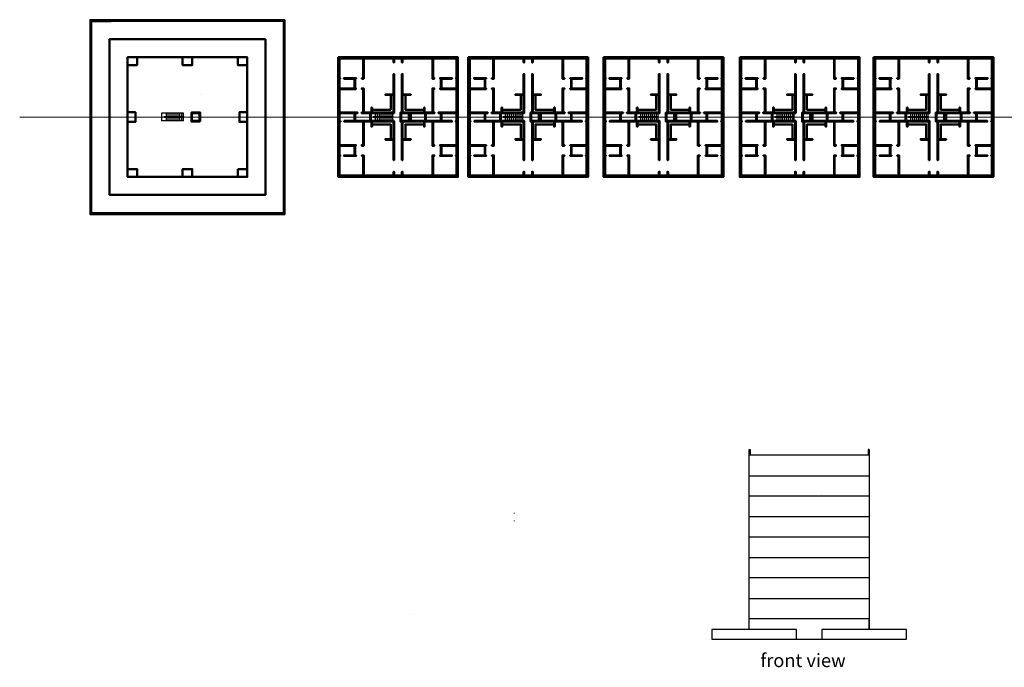
# Model space of a CAD drawing. Units: feet. Extents: x -1943 to 7856, y -1242 to 2749.
# Tile 1 of 2: x -1943 to 4124, y -1242 to 2749. Entities that reach past the tile are written whole.
import ezdxf

# ---------------------------------------------------------------- set-up
doc = ezdxf.new("R2010")
doc.units = ezdxf.units.FT
for name, color, linetype, lineweight in [('A-ANNO-SYMB', 1, 'Continuous', 18), ('A-ANNO-TEXT', 7, 'Continuous', 25), ('A-CONS', 8, 'Continuous', 13), ('A-ELEV', 7, 'Continuous', 25), ('A-FLOR-STRS', 3, 'Continuous', 25), ('A-WALL', 7, 'Continuous', 50), ('C-PROP', 6, 'Continuous', 35)]:
    doc.layers.add(name, color=color, linetype=linetype, lineweight=lineweight)
doc.styles.get("Standard").update_dxf_attribs({"font": 'arial.ttf'})

# ---------------------------------------------------------------- blocks, each defined once
blk = doc.blocks.new('STAIR')
for p, q in [((-933.2, 2172.8), (-1068.1, 2172.8)), ((-1068.1, 2172.8), (-1068.1, 2124.8)), ((-933.2, 2124.8), (-1068.1, 2124.8)), ((-1041.2, 2172.8), (-1041.2, 2151.4)), ((-1041.2, 2146.3), (-1041.2, 2124.8)), ((-1029.2, 2172.8), (-1029.2, 2151.4)), ((-1029.2, 2146.3), (-1029.2, 2124.8)), ((-1017.2, 2172.8), (-1017.2, 2151.4)), ((-1017.2, 2146.3), (-1017.2, 2124.8)), ((-1005.2, 2172.8), (-1005.2, 2151.4)), ((-1005.2, 2146.3), (-1005.2, 2124.8)), ((-993.2, 2172.8), (-993.2, 2151.4)), ((-993.2, 2146.3), (-993.2, 2124.8)), ((-981.2, 2172.8), (-981.2, 2151.4)), ((-981.2, 2146.3), (-981.2, 2124.8)), ((-969.2, 2172.8), (-969.2, 2151.4)), ((-969.2, 2146.3), (-969.2, 2124.8)), ((-957.2, 2172.8), (-957.2, 2151.4)), ((-957.2, 2146.3), (-957.2, 2124.8)), ((-945.2, 2172.8), (-945.2, 2151.4))]:
    blk.add_line(p, q)
for points in [[(-1053.2, 2151.4), (-933.2, 2151.4), (-933.2, 2146.3), (-1053.2, 2146.3)], [(-1052.2, 2150.4), (-934.2, 2150.4), (-934.2, 2147.3), (-1052.2, 2147.3)]]:
    blk.add_lwpolyline(points, close=True)
for points in [[(-945.2, 2146.3), (-945.2, 2124.8)], [(-933.2, 2124.8), (-933.2, 2172.8)]]:
    blk.add_lwpolyline(points)

msp = doc.modelspace()

# ---------------------------------------------------------------- linework, layer by layer
at = {"layer": 'A-ANNO-SYMB'}
msp.add_line((-1942.9, 2148.8), (7856.1, 2148.8), dxfattribs=at)
at = {"layer": 'A-CONS'}
for p, q in [((1105.6, -291.9, 260.8), (1101.6, -291.9, 260.8)), ((1105.6, -339.9, 260.8), (1101.6, -339.9, 260.8)), ((477.6, -915.9, 80.8), (477.6, -915.9, 140.8))]:
    msp.add_line(p, q, dxfattribs=at)
at = {"layer": 'A-ELEV'}
for p, q in [((2552.9, 100.4), (2558.9, 100.4)), ((2552.9, -1009.6), (2552.9, 100.4)), ((3290.9, 64.4), (2552.9, 64.4)), ((2558.9, 100.4), (2558.9, 64.4)), ((3290.9, 100.4), (3284.9, 100.4)), ((3284.9, 100.4), (3284.9, 64.4)), ((3290.9, 64.4), (3290.9, 100.4)), ((3290.9, 100.4), (3290.9, -1009.6)), ((2552.9, -61.6), (3290.9, -61.6)), ((3000, -175.9), (3000, -175.9)), ((3290.9, -187.6), (2552.9, -187.6)), ((2552.9, -313.6), (3290.9, -313.6)), ((3290.9, -439.6), (2552.9, -439.6)), ((3290.9, -439.6), (2552.9, -439.6)), ((2552.9, -565.6), (3290.9, -565.6)), ((3290.9, -691.6), (2552.9, -691.6)), ((2552.9, -817.6), (3290.9, -817.6)), ((3290.9, -943.6), (2552.9, -943.6)), ((3290.9, -1009.6), (3290.9, -949.6)), ((2844.1, -1009.6), (2321.9, -1009.6)), ((2321.9, -1009.6), (2321.9, -1069.6)), ((2844.1, -1069.6), (2844.1, -1009.6)), ((3521.9, -1009.6), (2999.8, -1009.6)), ((2999.8, -1009.6), (2999.8, -1069.6)), ((3521.9, -1069.6), (3521.9, -1009.6)), ((2321.9, -1069.6), (3521.9, -1069.6))]:
    msp.add_line(p, q, dxfattribs=at)
at = {"layer": 'A-WALL'}
for p, q in [((-1500.2, 2739.8), (-1380.2, 2739.8)), ((-1389.2, 2628.8), (-429.2, 2628.8)), ((-1389.2, 1668.8), (-1389.2, 2628.8)), ((-429.2, 2628.8), (-429.2, 1668.8)), ((-831.1, 2288.8), (-831.1, 2288.8)), ((466.6, 2288.8), (466.6, 2288.8)), ((1268.5, 2288.8), (1268.5, 2288.8)), ((2102.6, 2288.8), (2102.6, 2288.8)), ((2941.6, 2288.8), (2941.6, 2288.8)), ((3766, 2288.8), (3766, 2288.8)), ((-429.2, 1668.8), (-1389.2, 1668.8))]:
    msp.add_line(p, q, dxfattribs=at)
for points in [[(-429.2, 2628.8), (-429.2, 1668.8), (-1389.2, 1668.8), (-1389.2, 2628.8)], [(-540.2, 2517.8), (-540.2, 1779.8), (-1278.2, 1779.8), (-1278.2, 2517.8)], [(-1278.2, 2517.8), (-1219.1, 2517.8), (-1219.1, 2469.1), (-1278.2, 2469.1)], [(-938.7, 2517.8), (-879.6, 2517.8), (-879.6, 2469.1), (-938.7, 2469.1)], [(-599.2, 2517.8), (-540.2, 2517.8), (-540.2, 2469.1), (-599.2, 2469.1)], [(19.6, 2517.8), (19.6, 1779.8), (757.6, 1779.8), (757.6, 2517.8)], [(821.4, 2517.8), (821.4, 1779.8), (1559.4, 1779.8), (1559.4, 2517.8)], [(1655.5, 2517.8), (1655.5, 1779.8), (2393.5, 1779.8), (2393.5, 2517.8)], [(2494.5, 2517.8), (2494.5, 1779.8), (3232.5, 1779.8), (3232.5, 2517.8)], [(3319, 2517.8), (3319, 1779.8), (4057, 1779.8), (4057, 2517.8)], [(-1278.2, 2119.3), (-1278.2, 2178.4), (-1229.4, 2178.4), (-1229.4, 2119.3)], [(-830.6, 2120.8), (-885.2, 2120.8), (-885.2, 2176.8), (-830.6, 2176.8)], [(-834.6, 2124.8), (-881.2, 2124.8), (-881.2, 2172.8), (-834.6, 2172.8)], [(-540.2, 2178.4), (-540.2, 2119.3), (-588.9, 2119.3), (-588.9, 2178.4)], [(458.1, 2120.8), (403.5, 2120.8), (403.5, 2176.8), (458.1, 2176.8)], [(454.1, 2124.8), (407.5, 2124.8), (407.5, 2172.8), (454.1, 2172.8)], [(1260, 2120.8), (1205.3, 2120.8), (1205.3, 2176.8), (1260, 2176.8)], [(1256, 2124.8), (1209.3, 2124.8), (1209.3, 2172.8), (1256, 2172.8)], [(2094.1, 2120.8), (2039.5, 2120.8), (2039.5, 2176.8), (2094.1, 2176.8)], [(2090.1, 2124.8), (2043.5, 2124.8), (2043.5, 2172.8), (2090.1, 2172.8)], [(2933.1, 2120.8), (2878.5, 2120.8), (2878.5, 2176.8), (2933.1, 2176.8)], [(2929.1, 2124.8), (2882.5, 2124.8), (2882.5, 2172.8), (2929.1, 2172.8)], [(3757.5, 2120.8), (3702.9, 2120.8), (3702.9, 2176.8), (3757.5, 2176.8)], [(3753.5, 2124.8), (3706.9, 2124.8), (3706.9, 2172.8), (3753.5, 2172.8)], [(-1278.2, 1828.6), (-1219.1, 1828.6), (-1219.1, 1779.8), (-1278.2, 1779.8)], [(-879.6, 1779.8), (-938.7, 1779.8), (-938.7, 1828.6), (-879.6, 1828.6)], [(-599.2, 1828.6), (-540.2, 1828.6), (-540.2, 1779.8), (-599.2, 1779.8)]]:
    msp.add_lwpolyline(points, close=True, dxfattribs=at)
for points in [[(560.6, 2124.8), (652.6, 2124.8), (652.6, 2172.8), (637.7, 2172.8), (637.7, 2176.8), (748.6, 2176.8), (748.6, 2321.3), (647.8, 2321.3), (647.8, 2325.3), (652.6, 2325.3), (652.6, 2384.8), (647.5, 2384.8), (647.5, 2388.8), (722, 2388.8), (722, 2384.8), (656.6, 2384.8), (656.6, 2325.3), (748.6, 2325.3), (748.6, 2384.8), (746, 2384.8), (746, 2388.8), (748.6, 2388.8), (748.6, 2508.8), (604.1, 2508.8), (604.1, 2388.8), (611.5, 2388.8), (611.5, 2384.8), (600.1, 2384.8), (600.1, 2508.8), (416.6, 2508.8), (416.6, 2485.7), (412.6, 2485.7), (412.6, 2508.8), (364.6, 2508.8), (364.6, 2485.7), (360.6, 2485.7), (360.6, 2508.8), (177.1, 2508.8), (177.1, 2384.8), (165.6, 2384.8), (165.6, 2388.8), (173.1, 2388.8), (173.1, 2508.8), (28.6, 2508.8), (28.6, 2388.8), (31.1, 2388.8), (31.1, 2384.8), (28.6, 2384.8), (28.6, 2325.3), (120.6, 2325.3), (120.6, 2384.8), (55.1, 2384.8), (55.1, 2388.8), (129.6, 2388.8), (129.6, 2384.8), (124.6, 2384.8), (124.6, 2325.3), (129.4, 2325.3), (129.4, 2321.3), (28.6, 2321.3), (28.6, 2176.8), (139.5, 2176.8), (139.5, 2172.8), (124.6, 2172.8), (124.6, 2124.8), (216.6, 2124.8), (216.6, 2172.8), (216.6, 2124.8), (216.6, 2172.8), (163.5, 2172.8), (163.5, 2176.8), (173.1, 2176.8), (173.1, 2321.3), (165.4, 2321.3), (165.4, 2325.3), (177.1, 2325.3), (177.1, 2176.8), (224.6, 2176.8), (224.6, 2207.4), (228.6, 2207.4), (228.6, 2176.8), (360.6, 2176.8), (360.6, 2284.8), (310.5, 2284.8), (310.5, 2288.8), (360.6, 2288.8), (360.6, 2413.7), (364.6, 2413.7), (364.6, 2172.8), (220.6, 2172.8), (220.6, 2124.8), (364.6, 2124.8), (364.6, 1884), (360.6, 1884), (360.6, 2008.8), (310.5, 2008.8), (310.5, 2012.8), (360.6, 2012.8), (360.6, 2120.8), (228.6, 2120.8), (228.6, 2090.3), (224.6, 2090.3), (224.6, 2120.8), (177.1, 2120.8), (177.1, 1972.3), (165.4, 1972.3), (165.4, 1976.3), (173.1, 1976.3), (173.1, 2120.8), (57.1, 2120.8), (57.1, 2124.8), (120.6, 2124.8), (120.6, 2172.8), (28.6, 2172.8), (28.6, 2124.8), (33.1, 2124.8), (33.1, 2120.8), (28.6, 2120.8), (28.6, 1976.3), (129.4, 1976.3), (129.4, 1972.3), (124.6, 1972.3), (124.6, 1912.8), (129.6, 1912.8), (129.6, 1908.8), (56.5, 1908.8), (56.5, 1912.8), (120.6, 1912.8), (120.6, 1972.3), (28.6, 1972.3), (28.6, 1912.8), (32.5, 1912.8), (32.5, 1908.8), (28.6, 1908.8), (28.6, 1788.8), (173.1, 1788.8), (173.1, 1908.8), (165.6, 1908.8), (165.6, 1912.8), (177.1, 1912.8), (177.1, 1788.8), (360.6, 1788.8), (360.6, 1812), (364.6, 1812), (364.6, 1788.8), (412.6, 1788.8), (412.6, 1812), (416.6, 1812), (416.6, 1788.8), (600.1, 1788.8), (600.1, 1912.8), (611.5, 1912.8), (611.5, 1908.8), (604.1, 1908.8), (604.1, 1788.8), (748.6, 1788.8), (748.6, 1908.8), (744.7, 1908.8), (744.7, 1912.8), (748.6, 1912.8), (748.6, 1972.3), (656.6, 1972.3), (656.6, 1912.8), (720.7, 1912.8), (720.7, 1908.8), (647.5, 1908.8), (647.5, 1912.8), (652.6, 1912.8), (652.6, 1972.3), (647.8, 1972.3), (647.8, 1976.3), (748.6, 1976.3), (748.6, 2120.8), (744.1, 2120.8), (744.1, 2124.8), (748.6, 2124.8), (748.6, 2172.8), (656.6, 2172.8), (656.6, 2124.8), (720.1, 2124.8), (720.1, 2120.8), (604.1, 2120.8), (604.1, 1976.3), (611.8, 1976.3), (611.8, 1972.3), (600.1, 1972.3), (600.1, 2120.8), (552.6, 2120.8), (552.6, 2090.3), (548.6, 2090.3), (548.6, 2120.8), (416.6, 2120.8), (416.6, 2012.8), (466.6, 2012.8), (466.6, 2008.8), (416.6, 2008.8), (416.6, 1884), (412.6, 1884), (412.6, 2124.8), (463.2, 2124.8), (463.2, 2172.8), (412.6, 2172.8), (412.6, 2413.7), (416.6, 2413.7), (416.6, 2288.8), (466.6, 2288.8), (466.6, 2284.8), (416.6, 2284.8), (416.6, 2176.8), (548.6, 2176.8), (548.6, 2207.4), (552.6, 2207.4), (552.6, 2176.8), (600.1, 2176.8), (600.1, 2325.3), (611.8, 2325.3), (611.8, 2321.3), (604.1, 2321.3), (604.1, 2176.8), (613.7, 2176.8), (613.7, 2172.8), (560.6, 2172.8), (560.6, 2124.8), (560.6, 2172.8)], [(1362.4, 2124.8), (1454.4, 2124.8), (1454.4, 2172.8), (1439.5, 2172.8), (1439.5, 2176.8), (1550.4, 2176.8), (1550.4, 2321.3), (1449.6, 2321.3), (1449.6, 2325.3), (1454.4, 2325.3), (1454.4, 2384.8), (1449.3, 2384.8), (1449.3, 2388.8), (1523.8, 2388.8), (1523.8, 2384.8), (1458.4, 2384.8), (1458.4, 2325.3), (1550.4, 2325.3), (1550.4, 2384.8), (1547.8, 2384.8), (1547.8, 2388.8), (1550.4, 2388.8), (1550.4, 2508.8), (1405.9, 2508.8), (1405.9, 2388.8), (1413.3, 2388.8), (1413.3, 2384.8), (1401.9, 2384.8), (1401.9, 2508.8), (1218.4, 2508.8), (1218.4, 2485.7), (1214.4, 2485.7), (1214.4, 2508.8), (1166.4, 2508.8), (1166.4, 2485.7), (1162.4, 2485.7), (1162.4, 2508.8), (978.9, 2508.8), (978.9, 2384.8), (967.4, 2384.8), (967.4, 2388.8), (974.9, 2388.8), (974.9, 2508.8), (830.4, 2508.8), (830.4, 2388.8), (832.9, 2388.8), (832.9, 2384.8), (830.4, 2384.8), (830.4, 2325.3), (922.4, 2325.3), (922.4, 2384.8), (856.9, 2384.8), (856.9, 2388.8), (931.4, 2388.8), (931.4, 2384.8), (926.4, 2384.8), (926.4, 2325.3), (931.2, 2325.3), (931.2, 2321.3), (830.4, 2321.3), (830.4, 2176.8), (941.3, 2176.8), (941.3, 2172.8), (926.4, 2172.8), (926.4, 2124.8), (1018.4, 2124.8), (1018.4, 2172.8), (1018.4, 2124.8), (1018.4, 2172.8), (965.3, 2172.8), (965.3, 2176.8), (974.9, 2176.8), (974.9, 2321.3), (967.2, 2321.3), (967.2, 2325.3), (978.9, 2325.3), (978.9, 2176.8), (1026.4, 2176.8), (1026.4, 2207.4), (1030.4, 2207.4), (1030.4, 2176.8), (1162.4, 2176.8), (1162.4, 2284.8), (1112.3, 2284.8), (1112.3, 2288.8), (1162.4, 2288.8), (1162.4, 2413.7), (1166.4, 2413.7), (1166.4, 2172.8), (1022.4, 2172.8), (1022.4, 2124.8), (1166.4, 2124.8), (1166.4, 1884), (1162.4, 1884), (1162.4, 2008.8), (1112.3, 2008.8), (1112.3, 2012.8), (1162.4, 2012.8), (1162.4, 2120.8), (1030.4, 2120.8), (1030.4, 2090.3), (1026.4, 2090.3), (1026.4, 2120.8), (978.9, 2120.8), (978.9, 1972.3), (967.2, 1972.3), (967.2, 1976.3), (974.9, 1976.3), (974.9, 2120.8), (858.9, 2120.8), (858.9, 2124.8), (922.4, 2124.8), (922.4, 2172.8), (830.4, 2172.8), (830.4, 2124.8), (834.9, 2124.8), (834.9, 2120.8), (830.4, 2120.8), (830.4, 1976.3), (931.2, 1976.3), (931.2, 1972.3), (926.4, 1972.3), (926.4, 1912.8), (931.4, 1912.8), (931.4, 1908.8), (858.3, 1908.8), (858.3, 1912.8), (922.4, 1912.8), (922.4, 1972.3), (830.4, 1972.3), (830.4, 1912.8), (834.3, 1912.8), (834.3, 1908.8), (830.4, 1908.8), (830.4, 1788.8), (974.9, 1788.8), (974.9, 1908.8), (967.4, 1908.8), (967.4, 1912.8), (978.9, 1912.8), (978.9, 1788.8), (1162.4, 1788.8), (1162.4, 1812), (1166.4, 1812), (1166.4, 1788.8), (1214.4, 1788.8), (1214.4, 1812), (1218.4, 1812), (1218.4, 1788.8), (1401.9, 1788.8), (1401.9, 1912.8), (1413.3, 1912.8), (1413.3, 1908.8), (1405.9, 1908.8), (1405.9, 1788.8), (1550.4, 1788.8), (1550.4, 1908.8), (1546.5, 1908.8), (1546.5, 1912.8), (1550.4, 1912.8), (1550.4, 1972.3), (1458.4, 1972.3), (1458.4, 1912.8), (1522.5, 1912.8), (1522.5, 1908.8), (1449.3, 1908.8), (1449.3, 1912.8), (1454.4, 1912.8), (1454.4, 1972.3), (1449.6, 1972.3), (1449.6, 1976.3), (1550.4, 1976.3), (1550.4, 2120.8), (1545.9, 2120.8), (1545.9, 2124.8), (1550.4, 2124.8), (1550.4, 2172.8), (1458.4, 2172.8), (1458.4, 2124.8), (1521.9, 2124.8), (1521.9, 2120.8), (1405.9, 2120.8), (1405.9, 1976.3), (1413.6, 1976.3), (1413.6, 1972.3), (1401.9, 1972.3), (1401.9, 2120.8), (1354.4, 2120.8), (1354.4, 2090.3), (1350.4, 2090.3), (1350.4, 2120.8), (1218.4, 2120.8), (1218.4, 2012.8), (1268.5, 2012.8), (1268.5, 2008.8), (1218.4, 2008.8), (1218.4, 1884), (1214.4, 1884), (1214.4, 2124.8), (1265, 2124.8), (1265, 2172.8), (1214.4, 2172.8), (1214.4, 2413.7), (1218.4, 2413.7), (1218.4, 2288.8), (1268.5, 2288.8), (1268.5, 2284.8), (1218.4, 2284.8), (1218.4, 2176.8), (1350.4, 2176.8), (1350.4, 2207.4), (1354.4, 2207.4), (1354.4, 2176.8), (1401.9, 2176.8), (1401.9, 2325.3), (1413.6, 2325.3), (1413.6, 2321.3), (1405.9, 2321.3), (1405.9, 2176.8), (1415.5, 2176.8), (1415.5, 2172.8), (1362.4, 2172.8), (1362.4, 2124.8), (1362.4, 2172.8)], [(2196.5, 2124.8), (2288.5, 2124.8), (2288.5, 2172.8), (2273.6, 2172.8), (2273.6, 2176.8), (2384.5, 2176.8), (2384.5, 2321.3), (2283.7, 2321.3), (2283.7, 2325.3), (2288.5, 2325.3), (2288.5, 2384.8), (2283.5, 2384.8), (2283.5, 2388.8), (2358, 2388.8), (2358, 2384.8), (2292.5, 2384.8), (2292.5, 2325.3), (2384.5, 2325.3), (2384.5, 2384.8), (2382, 2384.8), (2382, 2388.8), (2384.5, 2388.8), (2384.5, 2508.8), (2240, 2508.8), (2240, 2388.8), (2247.5, 2388.8), (2247.5, 2384.8), (2236, 2384.8), (2236, 2508.8), (2052.5, 2508.8), (2052.5, 2485.7), (2048.5, 2485.7), (2048.5, 2508.8), (2000.5, 2508.8), (2000.5, 2485.7), (1996.5, 2485.7), (1996.5, 2508.8), (1813, 2508.8), (1813, 2384.8), (1801.6, 2384.8), (1801.6, 2388.8), (1809, 2388.8), (1809, 2508.8), (1664.5, 2508.8), (1664.5, 2388.8), (1667.1, 2388.8), (1667.1, 2384.8), (1664.5, 2384.8), (1664.5, 2325.3), (1756.5, 2325.3), (1756.5, 2384.8), (1691.1, 2384.8), (1691.1, 2388.8), (1765.6, 2388.8), (1765.6, 2384.8), (1760.5, 2384.8), (1760.5, 2325.3), (1765.4, 2325.3), (1765.4, 2321.3), (1664.5, 2321.3), (1664.5, 2176.8), (1775.4, 2176.8), (1775.4, 2172.8), (1760.5, 2172.8), (1760.5, 2124.8), (1852.5, 2124.8), (1852.5, 2172.8), (1852.5, 2124.8), (1852.5, 2172.8), (1799.4, 2172.8), (1799.4, 2176.8), (1809, 2176.8), (1809, 2321.3), (1801.4, 2321.3), (1801.4, 2325.3), (1813, 2325.3), (1813, 2176.8), (1860.5, 2176.8), (1860.5, 2207.4), (1864.5, 2207.4), (1864.5, 2176.8), (1996.5, 2176.8), (1996.5, 2284.8), (1946.5, 2284.8), (1946.5, 2288.8), (1996.5, 2288.8), (1996.5, 2413.7), (2000.5, 2413.7), (2000.5, 2172.8), (1856.5, 2172.8), (1856.5, 2124.8), (2000.5, 2124.8), (2000.5, 1884), (1996.5, 1884), (1996.5, 2008.8), (1946.5, 2008.8), (1946.5, 2012.8), (1996.5, 2012.8), (1996.5, 2120.8), (1864.5, 2120.8), (1864.5, 2090.3), (1860.5, 2090.3), (1860.5, 2120.8), (1813, 2120.8), (1813, 1972.3), (1801.4, 1972.3), (1801.4, 1976.3), (1809, 1976.3), (1809, 2120.8), (1693, 2120.8), (1693, 2124.8), (1756.5, 2124.8), (1756.5, 2172.8), (1664.5, 2172.8), (1664.5, 2124.8), (1669, 2124.8), (1669, 2120.8), (1664.5, 2120.8), (1664.5, 1976.3), (1765.4, 1976.3), (1765.4, 1972.3), (1760.5, 1972.3), (1760.5, 1912.8), (1765.6, 1912.8), (1765.6, 1908.8), (1692.4, 1908.8), (1692.4, 1912.8), (1756.5, 1912.8), (1756.5, 1972.3), (1664.5, 1972.3), (1664.5, 1912.8), (1668.4, 1912.8), (1668.4, 1908.8), (1664.5, 1908.8), (1664.5, 1788.8), (1809, 1788.8), (1809, 1908.8), (1801.6, 1908.8), (1801.6, 1912.8), (1813, 1912.8), (1813, 1788.8), (1996.5, 1788.8), (1996.5, 1812), (2000.5, 1812), (2000.5, 1788.8), (2048.5, 1788.8), (2048.5, 1812), (2052.5, 1812), (2052.5, 1788.8), (2236, 1788.8), (2236, 1912.8), (2247.5, 1912.8), (2247.5, 1908.8), (2240, 1908.8), (2240, 1788.8), (2384.5, 1788.8), (2384.5, 1908.8), (2380.6, 1908.8), (2380.6, 1912.8), (2384.5, 1912.8), (2384.5, 1972.3), (2292.5, 1972.3), (2292.5, 1912.8), (2356.6, 1912.8), (2356.6, 1908.8), (2283.5, 1908.8), (2283.5, 1912.8), (2288.5, 1912.8), (2288.5, 1972.3), (2283.7, 1972.3), (2283.7, 1976.3), (2384.5, 1976.3), (2384.5, 2120.8), (2380, 2120.8), (2380, 2124.8), (2384.5, 2124.8), (2384.5, 2172.8), (2292.5, 2172.8), (2292.5, 2124.8), (2356, 2124.8), (2356, 2120.8), (2240, 2120.8), (2240, 1976.3), (2247.7, 1976.3), (2247.7, 1972.3), (2236, 1972.3), (2236, 2120.8), (2188.5, 2120.8), (2188.5, 2090.3), (2184.5, 2090.3), (2184.5, 2120.8), (2052.5, 2120.8), (2052.5, 2012.8), (2102.6, 2012.8), (2102.6, 2008.8), (2052.5, 2008.8), (2052.5, 1884), (2048.5, 1884), (2048.5, 2124.8), (2099.1, 2124.8), (2099.1, 2172.8), (2048.5, 2172.8), (2048.5, 2413.7), (2052.5, 2413.7), (2052.5, 2288.8), (2102.6, 2288.8), (2102.6, 2284.8), (2052.5, 2284.8), (2052.5, 2176.8), (2184.5, 2176.8), (2184.5, 2207.4), (2188.5, 2207.4), (2188.5, 2176.8), (2236, 2176.8), (2236, 2325.3), (2247.7, 2325.3), (2247.7, 2321.3), (2240, 2321.3), (2240, 2176.8), (2249.6, 2176.8), (2249.6, 2172.8), (2196.5, 2172.8), (2196.5, 2124.8), (2196.5, 2172.8)], [(3035.5, 2124.8), (3127.5, 2124.8), (3127.5, 2172.8), (3112.6, 2172.8), (3112.6, 2176.8), (3223.5, 2176.8), (3223.5, 2321.3), (3122.7, 2321.3), (3122.7, 2325.3), (3127.5, 2325.3), (3127.5, 2384.8), (3122.5, 2384.8), (3122.5, 2388.8), (3197, 2388.8), (3197, 2384.8), (3131.5, 2384.8), (3131.5, 2325.3), (3223.5, 2325.3), (3223.5, 2384.8), (3221, 2384.8), (3221, 2388.8), (3223.5, 2388.8), (3223.5, 2508.8), (3079, 2508.8), (3079, 2388.8), (3086.5, 2388.8), (3086.5, 2384.8), (3075, 2384.8), (3075, 2508.8), (2891.5, 2508.8), (2891.5, 2485.7), (2887.5, 2485.7), (2887.5, 2508.8), (2839.5, 2508.8), (2839.5, 2485.7), (2835.5, 2485.7), (2835.5, 2508.8), (2652, 2508.8), (2652, 2384.8), (2640.6, 2384.8), (2640.6, 2388.8), (2648, 2388.8), (2648, 2508.8), (2503.5, 2508.8), (2503.5, 2388.8), (2506.1, 2388.8), (2506.1, 2384.8), (2503.5, 2384.8), (2503.5, 2325.3), (2595.5, 2325.3), (2595.5, 2384.8), (2530.1, 2384.8), (2530.1, 2388.8), (2604.6, 2388.8), (2604.6, 2384.8), (2599.5, 2384.8), (2599.5, 2325.3), (2604.4, 2325.3), (2604.4, 2321.3), (2503.5, 2321.3), (2503.5, 2176.8), (2614.4, 2176.8), (2614.4, 2172.8), (2599.5, 2172.8), (2599.5, 2124.8), (2691.5, 2124.8), (2691.5, 2172.8), (2691.5, 2124.8), (2691.5, 2172.8), (2638.4, 2172.8), (2638.4, 2176.8), (2648, 2176.8), (2648, 2321.3), (2640.4, 2321.3), (2640.4, 2325.3), (2652, 2325.3), (2652, 2176.8), (2699.5, 2176.8), (2699.5, 2207.4), (2703.5, 2207.4), (2703.5, 2176.8), (2835.5, 2176.8), (2835.5, 2284.8), (2785.5, 2284.8), (2785.5, 2288.8), (2835.5, 2288.8), (2835.5, 2413.7), (2839.5, 2413.7), (2839.5, 2172.8), (2695.5, 2172.8), (2695.5, 2124.8), (2839.5, 2124.8), (2839.5, 1884), (2835.5, 1884), (2835.5, 2008.8), (2785.5, 2008.8), (2785.5, 2012.8), (2835.5, 2012.8), (2835.5, 2120.8), (2703.5, 2120.8), (2703.5, 2090.3), (2699.5, 2090.3), (2699.5, 2120.8), (2652, 2120.8), (2652, 1972.3), (2640.4, 1972.3), (2640.4, 1976.3), (2648, 1976.3), (2648, 2120.8), (2532, 2120.8), (2532, 2124.8), (2595.5, 2124.8), (2595.5, 2172.8), (2503.5, 2172.8), (2503.5, 2124.8), (2508, 2124.8), (2508, 2120.8), (2503.5, 2120.8), (2503.5, 1976.3), (2604.4, 1976.3), (2604.4, 1972.3), (2599.5, 1972.3), (2599.5, 1912.8), (2604.6, 1912.8), (2604.6, 1908.8), (2531.4, 1908.8), (2531.4, 1912.8), (2595.5, 1912.8), (2595.5, 1972.3), (2503.5, 1972.3), (2503.5, 1912.8), (2507.4, 1912.8), (2507.4, 1908.8), (2503.5, 1908.8), (2503.5, 1788.8), (2648, 1788.8), (2648, 1908.8), (2640.6, 1908.8), (2640.6, 1912.8), (2652, 1912.8), (2652, 1788.8), (2835.5, 1788.8), (2835.5, 1812), (2839.5, 1812), (2839.5, 1788.8), (2887.5, 1788.8), (2887.5, 1812), (2891.5, 1812), (2891.5, 1788.8), (3075, 1788.8), (3075, 1912.8), (3086.5, 1912.8), (3086.5, 1908.8), (3079, 1908.8), (3079, 1788.8), (3223.5, 1788.8), (3223.5, 1908.8), (3219.6, 1908.8), (3219.6, 1912.8), (3223.5, 1912.8), (3223.5, 1972.3), (3131.5, 1972.3), (3131.5, 1912.8), (3195.6, 1912.8), (3195.6, 1908.8), (3122.5, 1908.8), (3122.5, 1912.8), (3127.5, 1912.8), (3127.5, 1972.3), (3122.7, 1972.3), (3122.7, 1976.3), (3223.5, 1976.3), (3223.5, 2120.8), (3219, 2120.8), (3219, 2124.8), (3223.5, 2124.8), (3223.5, 2172.8), (3131.5, 2172.8), (3131.5, 2124.8), (3195, 2124.8), (3195, 2120.8), (3079, 2120.8), (3079, 1976.3), (3086.7, 1976.3), (3086.7, 1972.3), (3075, 1972.3), (3075, 2120.8), (3027.5, 2120.8), (3027.5, 2090.3), (3023.5, 2090.3), (3023.5, 2120.8), (2891.5, 2120.8), (2891.5, 2012.8), (2941.6, 2012.8), (2941.6, 2008.8), (2891.5, 2008.8), (2891.5, 1884), (2887.5, 1884), (2887.5, 2124.8), (2938.1, 2124.8), (2938.1, 2172.8), (2887.5, 2172.8), (2887.5, 2413.7), (2891.5, 2413.7), (2891.5, 2288.8), (2941.6, 2288.8), (2941.6, 2284.8), (2891.5, 2284.8), (2891.5, 2176.8), (3023.5, 2176.8), (3023.5, 2207.4), (3027.5, 2207.4), (3027.5, 2176.8), (3075, 2176.8), (3075, 2325.3), (3086.7, 2325.3), (3086.7, 2321.3), (3079, 2321.3), (3079, 2176.8), (3088.6, 2176.8), (3088.6, 2172.8), (3035.5, 2172.8), (3035.5, 2124.8), (3035.5, 2172.8)], [(3860, 2124.8), (3952, 2124.8), (3952, 2172.8), (3937.1, 2172.8), (3937.1, 2176.8), (4048, 2176.8), (4048, 2321.3), (3947.1, 2321.3), (3947.1, 2325.3), (3952, 2325.3), (3952, 2384.8), (3946.9, 2384.8), (3946.9, 2388.8), (4021.4, 2388.8), (4021.4, 2384.8), (3956, 2384.8), (3956, 2325.3), (4048, 2325.3), (4048, 2384.8), (4045.4, 2384.8), (4045.4, 2388.8), (4048, 2388.8), (4048, 2508.8), (3903.5, 2508.8), (3903.5, 2388.8), (3910.9, 2388.8), (3910.9, 2384.8), (3899.5, 2384.8), (3899.5, 2508.8), (3716, 2508.8), (3716, 2485.7), (3712, 2485.7), (3712, 2508.8), (3664, 2508.8), (3664, 2485.7), (3660, 2485.7), (3660, 2508.8), (3476.5, 2508.8), (3476.5, 2384.8), (3465, 2384.8), (3465, 2388.8), (3472.5, 2388.8), (3472.5, 2508.8), (3328, 2508.8), (3328, 2388.8), (3330.5, 2388.8), (3330.5, 2384.8), (3328, 2384.8), (3328, 2325.3), (3420, 2325.3), (3420, 2384.8), (3354.5, 2384.8), (3354.5, 2388.8), (3429, 2388.8), (3429, 2384.8), (3424, 2384.8), (3424, 2325.3), (3428.8, 2325.3), (3428.8, 2321.3), (3328, 2321.3), (3328, 2176.8), (3438.8, 2176.8), (3438.8, 2172.8), (3424, 2172.8), (3424, 2124.8), (3516, 2124.8), (3516, 2172.8), (3516, 2124.8), (3516, 2172.8), (3462.8, 2172.8), (3462.8, 2176.8), (3472.5, 2176.8), (3472.5, 2321.3), (3464.8, 2321.3), (3464.8, 2325.3), (3476.5, 2325.3), (3476.5, 2176.8), (3524, 2176.8), (3524, 2207.4), (3528, 2207.4), (3528, 2176.8), (3660, 2176.8), (3660, 2284.8), (3609.9, 2284.8), (3609.9, 2288.8), (3660, 2288.8), (3660, 2413.7), (3664, 2413.7), (3664, 2172.8), (3520, 2172.8), (3520, 2124.8), (3664, 2124.8), (3664, 1884), (3660, 1884), (3660, 2008.8), (3609.9, 2008.8), (3609.9, 2012.8), (3660, 2012.8), (3660, 2120.8), (3528, 2120.8), (3528, 2090.3), (3524, 2090.3), (3524, 2120.8), (3476.5, 2120.8), (3476.5, 1972.3), (3464.8, 1972.3), (3464.8, 1976.3), (3472.5, 1976.3), (3472.5, 2120.8), (3356.5, 2120.8), (3356.5, 2124.8), (3420, 2124.8), (3420, 2172.8), (3328, 2172.8), (3328, 2124.8), (3332.5, 2124.8), (3332.5, 2120.8), (3328, 2120.8), (3328, 1976.3), (3428.8, 1976.3), (3428.8, 1972.3), (3424, 1972.3), (3424, 1912.8), (3429, 1912.8), (3429, 1908.8), (3355.9, 1908.8), (3355.9, 1912.8), (3420, 1912.8), (3420, 1972.3), (3328, 1972.3), (3328, 1912.8), (3331.9, 1912.8), (3331.9, 1908.8), (3328, 1908.8), (3328, 1788.8), (3472.5, 1788.8), (3472.5, 1908.8), (3465, 1908.8), (3465, 1912.8), (3476.5, 1912.8), (3476.5, 1788.8), (3660, 1788.8), (3660, 1812), (3664, 1812), (3664, 1788.8), (3712, 1788.8), (3712, 1812), (3716, 1812), (3716, 1788.8), (3899.5, 1788.8), (3899.5, 1912.8), (3910.9, 1912.8), (3910.9, 1908.8), (3903.5, 1908.8), (3903.5, 1788.8), (4048, 1788.8), (4048, 1908.8), (4044, 1908.8), (4044, 1912.8), (4048, 1912.8), (4048, 1972.3), (3956, 1972.3), (3956, 1912.8), (4020, 1912.8), (4020, 1908.8), (3946.9, 1908.8), (3946.9, 1912.8), (3952, 1912.8), (3952, 1972.3), (3947.1, 1972.3), (3947.1, 1976.3), (4048, 1976.3), (4048, 2120.8), (4043.5, 2120.8), (4043.5, 2124.8), (4048, 2124.8), (4048, 2172.8), (3956, 2172.8), (3956, 2124.8), (4019.5, 2124.8), (4019.5, 2120.8), (3903.5, 2120.8), (3903.5, 1976.3), (3911.1, 1976.3), (3911.1, 1972.3), (3899.5, 1972.3), (3899.5, 2120.8), (3852, 2120.8), (3852, 2090.3), (3848, 2090.3), (3848, 2120.8), (3716, 2120.8), (3716, 2012.8), (3766, 2012.8), (3766, 2008.8), (3716, 2008.8), (3716, 1884), (3712, 1884), (3712, 2124.8), (3762.6, 2124.8), (3762.6, 2172.8), (3712, 2172.8), (3712, 2413.7), (3716, 2413.7), (3716, 2288.8), (3766, 2288.8), (3766, 2284.8), (3716, 2284.8), (3716, 2176.8), (3848, 2176.8), (3848, 2207.4), (3852, 2207.4), (3852, 2176.8), (3899.5, 2176.8), (3899.5, 2325.3), (3911.1, 2325.3), (3911.1, 2321.3), (3903.5, 2321.3), (3903.5, 2176.8), (3913.1, 2176.8), (3913.1, 2172.8), (3860, 2172.8), (3860, 2124.8), (3860, 2172.8)], [(228.6, 2193.8), (343.6, 2193.8), (343.6, 2284.8)], [(548.6, 2193.8), (433.6, 2193.8), (433.6, 2284.8)], [(1030.4, 2193.8), (1145.4, 2193.8), (1145.4, 2284.8)], [(1350.4, 2193.8), (1235.4, 2193.8), (1235.4, 2284.8)], [(1864.5, 2193.8), (1979.6, 2193.8), (1979.6, 2284.8)], [(2184.5, 2193.8), (2069.5, 2193.8), (2069.5, 2284.8)], [(2703.5, 2193.8), (2818.5, 2193.8), (2818.5, 2284.8)], [(3023.5, 2193.8), (2908.5, 2193.8), (2908.5, 2284.8)], [(3528, 2193.8), (3643, 2193.8), (3643, 2284.8)], [(3848, 2193.8), (3732.9, 2193.8), (3732.9, 2284.8)], [(556.6, 2124.8), (467.2, 2124.8), (467.2, 2172.8), (556.6, 2172.8), (556.6, 2124.8), (556.6, 2172.8)], [(1358.4, 2124.8), (1269, 2124.8), (1269, 2172.8), (1358.4, 2172.8), (1358.4, 2124.8), (1358.4, 2172.8)], [(2192.5, 2124.8), (2103.1, 2124.8), (2103.1, 2172.8), (2192.5, 2172.8), (2192.5, 2124.8), (2192.5, 2172.8)], [(3031.5, 2124.8), (2942.1, 2124.8), (2942.1, 2172.8), (3031.5, 2172.8), (3031.5, 2124.8), (3031.5, 2172.8)], [(3856, 2124.8), (3766.6, 2124.8), (3766.6, 2172.8), (3856, 2172.8), (3856, 2124.8), (3856, 2172.8)], [(228.6, 2103.9), (343.6, 2103.9), (343.6, 2012.8)], [(548.6, 2103.9), (433.6, 2103.9), (433.6, 2012.8)], [(1030.4, 2103.9), (1145.4, 2103.9), (1145.4, 2012.8)], [(1350.4, 2103.9), (1235.4, 2103.9), (1235.4, 2012.8)], [(1864.5, 2103.9), (1979.6, 2103.9), (1979.6, 2012.8)], [(2184.5, 2103.9), (2069.5, 2103.9), (2069.5, 2012.8)], [(2703.5, 2103.9), (2818.5, 2103.9), (2818.5, 2012.8)], [(3023.5, 2103.9), (2908.5, 2103.9), (2908.5, 2012.8)], [(3528, 2103.9), (3643, 2103.9), (3643, 2012.8)], [(3848, 2103.9), (3732.9, 2103.9), (3732.9, 2012.8)]]:
    msp.add_lwpolyline(points, dxfattribs=at)
at = {"layer": 'C-PROP'}
for points in [[(-309.2, 2748.8), (-309.2, 1548.8), (-1509.2, 1548.8), (-1509.2, 2748.8)], [(-318.2, 2739.8), (-318.2, 1557.8), (-1500.2, 1557.8), (-1500.2, 2739.8)]]:
    msp.add_lwpolyline(points, close=True, dxfattribs=at)

# ---------------------------------------------------------------- block references
at = {"layer": 'A-FLOR-STRS'}
msp.add_blockref('STAIR', (0, 0), dxfattribs=at)
at = {"layer": 'A-FLOR-STRS', "rotation": 0.0020692431570244}
for p in [(1288.8, 0), (2090.6, 0), (2924.7, 0), (3763.7, 0), (4588.2, 0)]:
    msp.add_blockref('STAIR', p, dxfattribs=at)

# ---------------------------------------------------------------- texts
at = {"layer": 'A-ANNO-TEXT', "insert": (2620.8, -1158.5), "char_height": 82.37, "attachment_point": 1}
msp.add_mtext_dynamic_manual_height_columns('front view', width=36742.22, gutter_width=411.8, heights=[0], dxfattribs=at)

doc.saveas('drawing.dxf')
